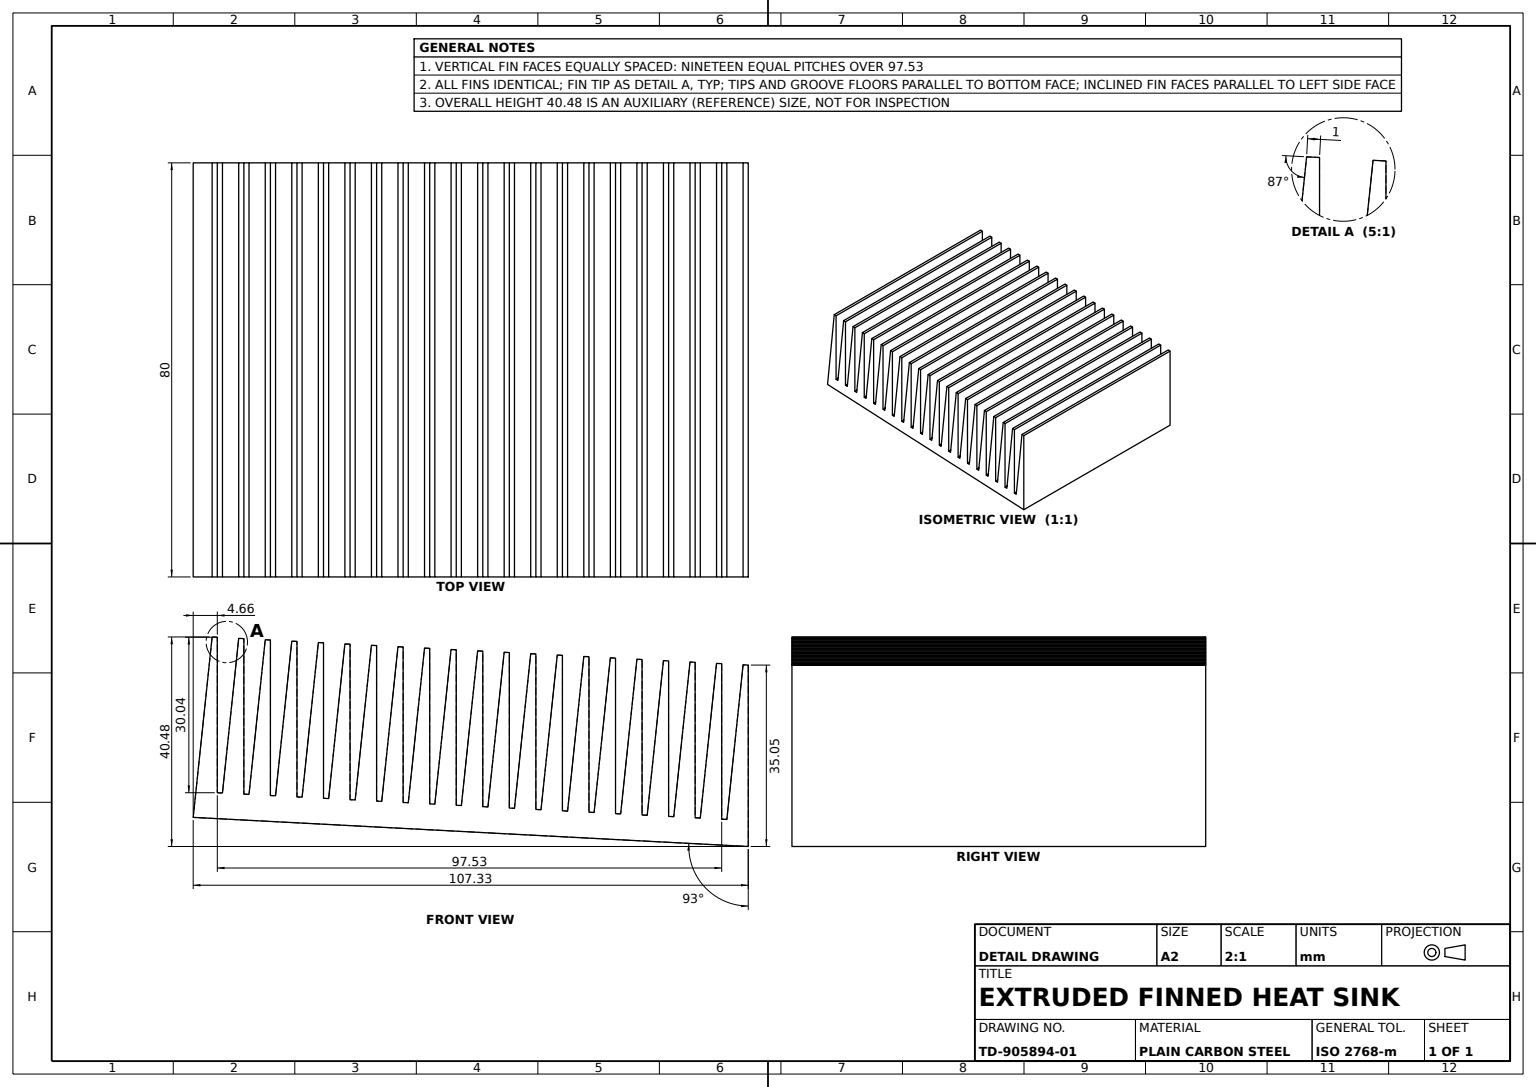
from build123d import *

# Parameters (mm, degrees)
HEAT_SINK_BODY_EXTRUDE_80MM_DEPTH = 80


with BuildPart() as part:
    # Heat Sink Profile 20 Fins → Heat Sink Body Extrude 80mm (new body)
    with BuildSketch(Plane(origin=(0, 0, 0), x_dir=(1, 0, 0), z_dir=(0, 1, 0))):
        Polygon((-38.997486194, 17.547966284), (-39.997486194, 17.547966284), (-41.831758469, -17.452033716), (65.641252838, -17.452033716), (63.806980563, 17.547966284), (62.806980563, 17.547966284), (61.234747185, -12.452033716), (60.239213942, -12.452033716), (58.666980563, 17.547966284), (57.666980563, 17.547966284), (56.094747185, -12.452033716), (55.099213942, -12.452033716), (53.526980563, 17.547966284), (52.526980563, 17.547966284), (50.954747185, -12.452033716), (49.959213942, -12.452033716), (48.386980563, 17.547966284), (47.386980563, 17.547966284), (45.814747185, -12.452033716), (44.819213942, -12.452033716), (43.246980563, 17.547966284), (42.246980563, 17.547966284), (40.674747185, -12.452033716), (39.679213942, -12.452033716), (38.106980563, 17.547966284), (37.106980563, 17.547966284), (35.534747185, -12.452033716), (34.539213942, -12.452033716), (32.966980563, 17.547966284), (31.966980563, 17.547966284), (30.394747185, -12.452033716), (29.399213942, -12.452033716), (27.826980563, 17.547966284), (26.826980563, 17.547966284), (25.254747185, -12.452033716), (24.259213942, -12.452033716), (22.686980563, 17.547966284), (21.686980563, 17.547966284), (20.114747185, -12.452033716), (19.119213942, -12.452033716), (17.546980563, 17.547966284), (16.546980563, 17.547966284), (14.974747185, -12.452033716), (13.979213942, -12.452033716), (12.406980563, 17.547966284), (11.406980563, 17.547966284), (9.834747185, -12.452033716), (8.839213942, -12.452033716), (7.266980563, 17.547966284), (6.266980563, 17.547966284), (4.694747185, -12.452033716), (3.699213942, -12.452033716), (2.126980563, 17.547966284), (1.126980563, 17.547966284), (-0.445252815, -12.452033716), (-1.440786058, -12.452033716), (-3.013019437, 17.547966284), (-4.013019437, 17.547966284), (-5.585252815, -12.452033716), (-6.580786058, -12.452033716), (-8.153019437, 17.547966284), (-9.153019437, 17.547966284), (-10.725252815, -12.452033716), (-11.720786058, -12.452033716), (-13.293019437, 17.547966284), (-13.392304127, 17.547966284), (-14.293019437, 17.547966284), (-15.865252815, -12.452033716), (-16.860786058, -12.452033716), (-18.433019437, 17.547966284), (-19.433019437, 17.547966284), (-21.005252815, -12.452033716), (-22.000786058, -12.452033716), (-23.573019437, 17.547966284), (-24.573019437, 17.547966284), (-26.145252815, -12.452033716), (-27.140786058, -12.452033716), (-28.713019437, 17.547966284), (-29.713019437, 17.547966284), (-31.285252815, -12.452033716), (-32.280786058, -12.452033716), (-33.853019437, 17.547966284), (-34.853019437, 17.547966284), (-36.425252815, -12.452033716), (-37.425252815, -12.452033716), align=None)
    extrude(amount=HEAT_SINK_BODY_EXTRUDE_80MM_DEPTH)


solid = part.part
